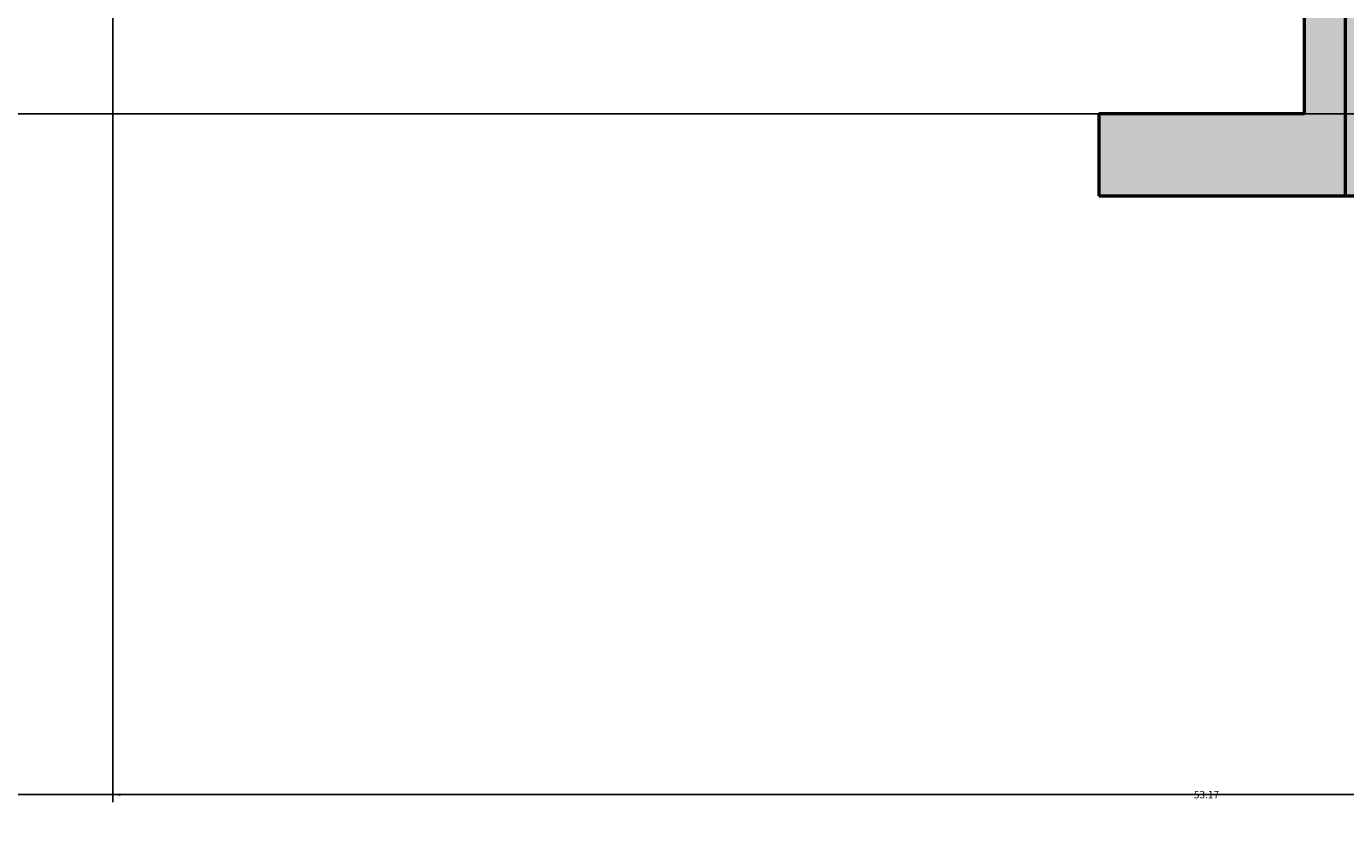
# Model space of a CAD drawing. Units: inches. Extents: x -12 to 334, y -10 to 186.
# Tile 11 of 77: x 74 to 106, y 13 to 33. Entities that reach past the tile are written whole.
import ezdxf
from ezdxf import colors
from ezdxf.entities.mleader import LeaderData, LeaderLine
from ezdxf.math import Vec2, Vec3

# ---------------------------------------------------------------- set-up
doc = ezdxf.new("R2010")
doc.units = ezdxf.units.IN
doc.header["$MEASUREMENT"] = 0
for name, color, linetype, lineweight in [('M-ANNO-TEXT', 3, 'Continuous', 25), ('M-DIMS', 2, 'Continuous', 18), ('M-EQPM', 7, 'Continuous', 50), ('M-EQPM-PATT', 8, 'Continuous', 18)]:
    doc.layers.add(name, color=color, linetype=linetype, lineweight=lineweight)
doc.styles.get("Standard").update_dxf_attribs({"font": 'arial.ttf'})
doc.dimstyles.get("Standard").update_dxf_attribs({"dimtxt": 0.18, "dimasz": 0.18, "dimexe": 0.18, "dimexo": 0.0625, "dimgap": 0.09, "dimtad": 0, "dimtih": 1, "dimtoh": 1, "dimdec": 4, "dimzin": 0, "dimdsep": 46, "dimtxsty": 'Standard', "dimcen": 0.09, "dimadec": 0, "dimazin": 0, "dimtfac": 1, "dimtdec": 4, "dimtofl": 0, "dimtmove": 0, "dimatfit": 3, "dimfxl": 1, "dimtolj": 1, "dimtzin": 0, "dimarcsym": 0})

# ---------------------------------------------------------------- blocks, each defined once
blk = doc.blocks.new('*D1')
at = {"layer": 'Defpoints', "color": 0, "transparency": 16777216}
for p in [(281.426, 91.899), (3.376, 80.692), (281.426, 14.304)]:
    blk.add_point(p, dxfattribs=at)
at = {"layer": 'M-DIMS', "color": 0, "lineweight": -2, "transparency": 16777216}
for p, q in [((281.426, 91.836), (281.426, 14.124)), ((3.376, 80.629), (3.376, 14.124)), ((3.556, 14.304), (141.935, 14.304)), ((281.246, 14.304), (142.867, 14.304))]:
    blk.add_line(p, q, dxfattribs=at)
at = {"layer": 'M-DIMS', "color": 0, "transparency": 16777216}
for points in [[(3.556, 14.334), (3.556, 14.274), (3.376, 14.304)], [(281.246, 14.334), (281.246, 14.274), (281.426, 14.304)]]:
    blk.add_solid(points, dxfattribs=at)
at = {"layer": 'M-DIMS', "color": 0, "transparency": 16777216, "insert": (142.401, 14.304), "char_height": 0.18, "attachment_point": 5}
blk.add_mtext('\\A1;278.05', dxfattribs=at)
blk = doc.blocks.new('*D29')
at = {"layer": 'Defpoints', "color": 0, "transparency": 16777216}
for p in [(-11.174, 45.854), (221.576, 45.854), (216.576, 30.854)]:
    blk.add_point(p, dxfattribs=at)
at = {"layer": 'M-DIMS', "color": 0, "lineweight": -2, "transparency": 16777216}
for p, q in [((221.514, 45.854), (-11.354, 45.854)), ((-11.174, 45.674), (-11.174, 38.536)), ((-11.174, 31.034), (-11.174, 38.172)), ((216.514, 30.854), (-11.354, 30.854))]:
    blk.add_line(p, q, dxfattribs=at)
at = {"layer": 'M-DIMS', "color": 0, "transparency": 16777216}
for points in [[(-11.204, 45.674), (-11.144, 45.674), (-11.174, 45.854)], [(-11.204, 31.034), (-11.144, 31.034), (-11.174, 30.854)]]:
    blk.add_solid(points, dxfattribs=at)
at = {"layer": 'M-DIMS', "color": 0, "transparency": 16777216, "insert": (-11.174, 38.354), "char_height": 0.18, "attachment_point": 5}
blk.add_mtext('\\A1;15', dxfattribs=at)
blk = doc.blocks.new('*D30')
at = {"layer": 'Defpoints', "color": 0, "transparency": 16777216}
for p in [(75.924, 63.612), (129.093, 61.105), (129.093, 14.304)]:
    blk.add_point(p, dxfattribs=at)
at = {"layer": 'M-DIMS', "color": 0, "lineweight": -2, "transparency": 16777216}
for p, q in [((75.924, 63.549), (75.924, 14.124)), ((129.093, 61.042), (129.093, 14.124)), ((76.104, 14.304), (102.115, 14.304)), ((128.913, 14.304), (102.902, 14.304))]:
    blk.add_line(p, q, dxfattribs=at)
at = {"layer": 'M-DIMS', "color": 0, "transparency": 16777216}
for points in [[(76.104, 14.334), (76.104, 14.274), (75.924, 14.304)], [(128.913, 14.334), (128.913, 14.274), (129.093, 14.304)]]:
    blk.add_solid(points, dxfattribs=at)
at = {"layer": 'M-DIMS', "color": 0, "transparency": 16777216, "insert": (102.509, 14.304), "char_height": 0.18, "attachment_point": 5}
blk.add_mtext('\\A1;53.17', dxfattribs=at)

msp = doc.modelspace()

# ---------------------------------------------------------------- hatches: boundary and pattern name
at = {"layer": 'M-EQPM-PATT'}
h = msp.add_hatch(color=256, dxfattribs=at)
h.set_gradient(color1=(99, 100, 102), color2=(99, 100, 102), tint=1)
h.paths.add_polyline_path([(4.3766, 80.754, -0.4132606), (23.5807, 99.8958), (37.1002, 99.8958), (37.1002, 127.7078), (32.1002, 127.7078), (32.1002, 125.2078), (36.1002, 125.2078), (36.1002, 100.8958), (23.5807, 100.8958, 1), (23.5807, 60.4872), (36.1002, 60.4872), (36.1002, 36.1752), (32.1002, 36.1752), (32.1002, 33.6752), (37.1002, 33.6752), (37.1002, 61.4872), (23.5807, 61.4872, -0.384914), (4.4744, 78.754), (72.9244, 78.754), (72.9244, 69.6117), (75.9244, 69.6117), (75.9244, 89.8963), (72.9244, 89.8963), (72.9244, 80.754)])
h.paths.add_polyline_path([(54.1002, 125.2078), (58.1002, 125.2078), (58.1002, 127.7078), (53.1002, 127.7078), (53.1002, 99.8958), (64.5, 99.8958), (64.5, 109.0583), (63.5, 109.0583), (63.5, 100.8958), (54.1002, 100.8958)], flags=17)
h.paths.add_polyline_path([(53.1002, 33.6752), (58.1002, 33.6752), (58.1002, 36.1752), (54.1002, 36.1752), (54.1002, 60.4872), (64.2068, 60.4872), (64.2068, 49.4497), (87.8879, 49.4497), (87.8879, 55.3205), (104.8919, 55.3205), (104.8919, 30.8541), (99.8919, 30.8541), (99.8919, 28.8541), (105.8919, 28.8541), (105.8919, 56.3205), (87.8879, 56.3205), (87.8879, 63.6117), (86.8879, 63.6117), (86.8879, 50.4497), (65.0061, 50.4497), (65.0061, 63.6117), (64.5, 63.6117), (64.5, 61.4872), (53.1002, 61.4872)])
h.paths.add_polyline_path([(121.8919, 28.8541), (121.8919, 30.8541), (116.8919, 30.8541), (116.8919, 45.8541), (209.6965, 45.8541), (209.9204, 46.8541), (115.8919, 46.8541), (115.8919, 28.8541)])
h.paths.add_polyline_path([(221.5761, 32.8541), (216.5761, 32.8541), (216.5761, 30.8541), (222.5761, 30.8541), (222.5761, 46.8541), (209.9204, 46.8541), (209.6965, 45.8541), (221.5761, 45.8541)])
h.paths.add_polyline_path([(233.5761, 45.8541), (249.8485, 45.8541), (249.3759, 46.8541), (232.5761, 46.8541), (232.5761, 30.8541), (238.5761, 30.8541), (238.5761, 32.8541), (233.5761, 32.8541)])
h = msp.add_hatch(color=256, dxfattribs=at)
h.set_gradient(color1=(94, 103, 175), color2=(94, 103, 175), tint=1)
h.paths.add_polyline_path([(129.093, 89.8963), (86.8879, 89.8963), (86.8879, 69.6117), (129.093, 69.6117)], flags=17)
h.paths.add_polyline_path([(170.9079, 89.8963), (130.8573, 89.8963), (130.8573, 69.6117), (170.9079, 69.6117)], flags=17)
h.paths.add_polyline_path([(216.4278, 89.8963), (172.6722, 89.8963), (172.6722, 69.6117), (216.4278, 69.6117)], flags=17)
h.paths.add_polyline_path([(245.9354, 82.6969), (247.9354, 82.6969), (247.9354, 46.8541), (268.3808, 46.8541, 0.0998398), (279.7263, 80.6915), (251.9801, 80.6915, 0.4142136), (231.7758, 100.8958), (84.7229, 100.8958), (84.7229, 109.0583), (83.7229, 109.0583), (83.7229, 95.8963), (129.093, 95.8963), (129.093, 98.1081), (130.8573, 98.1081), (130.8573, 95.8963), (170.9079, 95.8963), (170.9079, 98.1081), (172.6722, 98.1081), (172.6722, 95.8963), (216.4278, 95.8963), (216.4278, 98.1081), (218.1922, 98.1081), (218.1922, 95.8963), (226.6083, 95.8963, -1), (226.6083, 63.6117), (218.1922, 63.6117), (218.1922, 61.1045), (216.4278, 61.1045), (216.4278, 63.6117), (172.6722, 63.6117), (172.6722, 61.1045), (170.9079, 61.1045), (170.9079, 63.6117), (130.8573, 63.6117), (130.8573, 61.1045), (129.093, 61.1045), (129.093, 63.6117), (87.8879, 63.6117), (87.8879, 56.3205), (105.8919, 56.3205), (105.8919, 28.8541), (115.8919, 28.8541), (115.8919, 46.8541), (222.5761, 46.8541), (222.5761, 30.8541), (232.5761, 30.8541), (232.5761, 46.8541), (245.9354, 46.8541)])
h.paths.add_polyline_path([(86.8879, 89.8963), (75.9244, 89.8963), (75.9244, 69.6117), (86.8879, 69.6117)])
h.paths.add_polyline_path([(83.7229, 109.0583), (75.9244, 109.0583), (75.9244, 95.8963), (83.7229, 95.8963)])
h.paths.add_polyline_path([(226.6083, 89.8963), (218.1922, 89.8963), (218.1922, 69.6117), (226.6083, 69.6117, 1)], flags=17)
h = msp.add_hatch(color=256, dxfattribs=at)
h.set_gradient(color1=(0, 0, 255), color2=(0, 0, 255), tint=1)
h.paths.add_polyline_path([(84.7229, 100.8958), (84.7229, 109.0583), (83.7229, 109.0583), (83.7229, 95.8963), (129.093, 95.8963), (129.093, 98.1081), (130.8573, 98.1081), (130.8573, 95.8963), (170.9079, 95.8963), (170.9079, 98.1081), (172.6722, 98.1081), (172.6722, 95.8963), (216.4278, 95.8963), (216.4278, 98.1081), (218.1922, 98.1081), (218.1922, 95.8963), (226.6083, 95.8963, -1), (226.6083, 63.6117), (218.1922, 63.6117), (218.1922, 61.1045), (216.4278, 61.1045), (216.4278, 63.6117), (172.6722, 63.6117), (172.6722, 61.1045), (170.9079, 61.1045), (170.9079, 63.6117), (130.8573, 63.6117), (130.8573, 61.1045), (129.093, 61.1045), (129.093, 63.6117), (87.8879, 63.6117), (87.8879, 56.3205), (105.8919, 56.3205), (105.8919, 28.8541), (115.8919, 28.8541), (115.8919, 46.8541), (222.5761, 46.8541), (222.5761, 30.8541), (232.5761, 30.8541), (232.5761, 46.8541), (245.9354, 46.8541), (245.9354, 82.6969), (247.9354, 82.6969), (247.9354, 46.8541), (268.3808, 46.8541, 0.0998398), (279.7263, 80.6915), (251.9801, 80.6915, 0.4142136), (231.7758, 100.8958)])

# ---------------------------------------------------------------- linework, layer by layer
at = {"layer": 'M-EQPM'}
for p, q in [((105.8919, 28.8541), (105.8919, 56.3205)), ((104.8919, 30.8541), (104.8919, 55.3205)), ((104.8919, 30.8541), (99.8919, 30.8541)), ((99.8919, 30.8541), (99.8919, 28.8541)), ((99.8919, 28.8541), (121.8919, 28.8541))]:
    msp.add_line(p, q, dxfattribs=at)

# ---------------------------------------------------------------- dimensions: what is measured, and where the dimension line sits
at = {"layer": 'M-DIMS'}
for base, p1, p2, picture, middle in [((281.4256, 14.3041), (3.3765, 80.6915), (281.4256, 91.8988), '*D1', (142.401, 14.3041)), ((129.093, 14.3041), (75.9244, 63.6117), (129.093, 61.1045), '*D30', (102.5087, 14.3041))]:
    dim = msp.add_linear_dim(base=base, p1=p1, p2=p2, dimstyle='Standard', override={"dimdec": 2, "dimlfac": 1, "dimrnd": 0, "dimzin": 0, "dimdsep": 46, "dimlunit": 2}, dxfattribs=at)
    dim.commit()
    dim.dimension.update_dxf_attribs({"geometry": picture, "text_midpoint": middle})
dim = msp.add_linear_dim(base=(-11.1736, 45.8541), p1=(216.5761, 30.8541), p2=(221.5761, 45.8541), angle=90, dimstyle='Standard', override={"dimdec": 0, "dimlfac": 1, "dimrnd": 0, "dimzin": 0, "dimdsep": 46, "dimlunit": 2}, dxfattribs=at)
dim.commit()
dim.dimension.update_dxf_attribs({"geometry": '*D29', "text_midpoint": (-11.1735, 38.3541)})

# ---------------------------------------------------------------- leaders
at = {"layer": 'M-ANNO-TEXT'}
ml = msp.add_multileader_mtext('Standard', dxfattribs=at)
ml.set_content('^ICondensate outlet', color=256)
ml.set_leader_properties()
ml.build(insert=Vec2(0, 0))
ml.multileader.update_dxf_attribs({"dogleg_length": 0.36, "arrow_head_size": 0.7})
ctx = ml.context
ctx.base_point, ctx.arrow_head_size, ctx.landing_gap_size, ctx.plane_origin = Vec3(83.8784, 10.3512), 0.7, 0.09, Vec3(49.4251, 25.7584)
notes = []
notes.append((ctx, [(0, (1, 1, 0), (70.8242, 10.3512), (1, 0), 13.0542, [(0, [(42.9275, 33.6752)], 0, [])])]))
ctx.mtext.insert, ctx.mtext.flow_direction = Vec3(83.9684, 12.3853), 5
for ctx, leaders in notes:
    for number, flags, end, landing, length, lines in leaders:
        leader = LeaderData()
        leader.index, (leader.has_last_leader_line, leader.has_dogleg_vector, leader.attachment_direction) = number, flags
        leader.last_leader_point, leader.dogleg_vector, leader.dogleg_length = Vec3(end), Vec3(landing), length
        for number, points, colour, breaks in lines:
            line = LeaderLine()
            line.index, line.vertices, line.color, line.breaks = number, Vec3.list(points), colors.encode_raw_color(colour), breaks
            leader.lines.append(line)
        ctx.leaders.append(leader)

doc.saveas('drawing.dxf')
